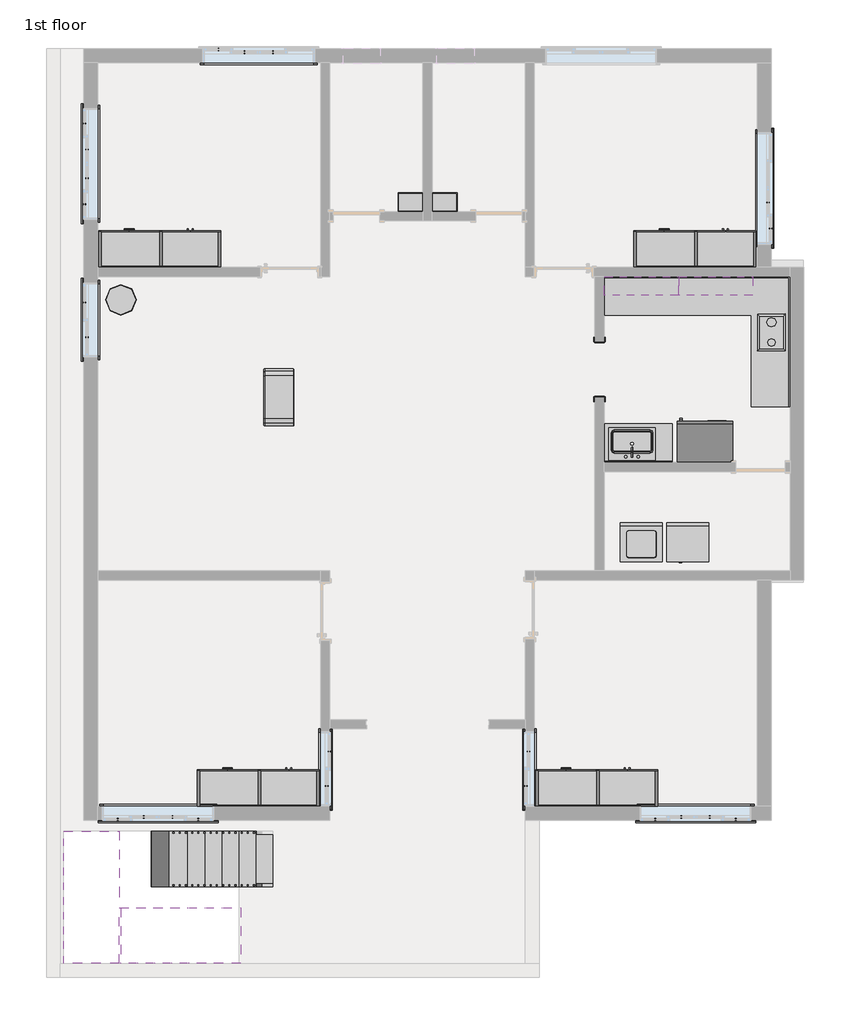
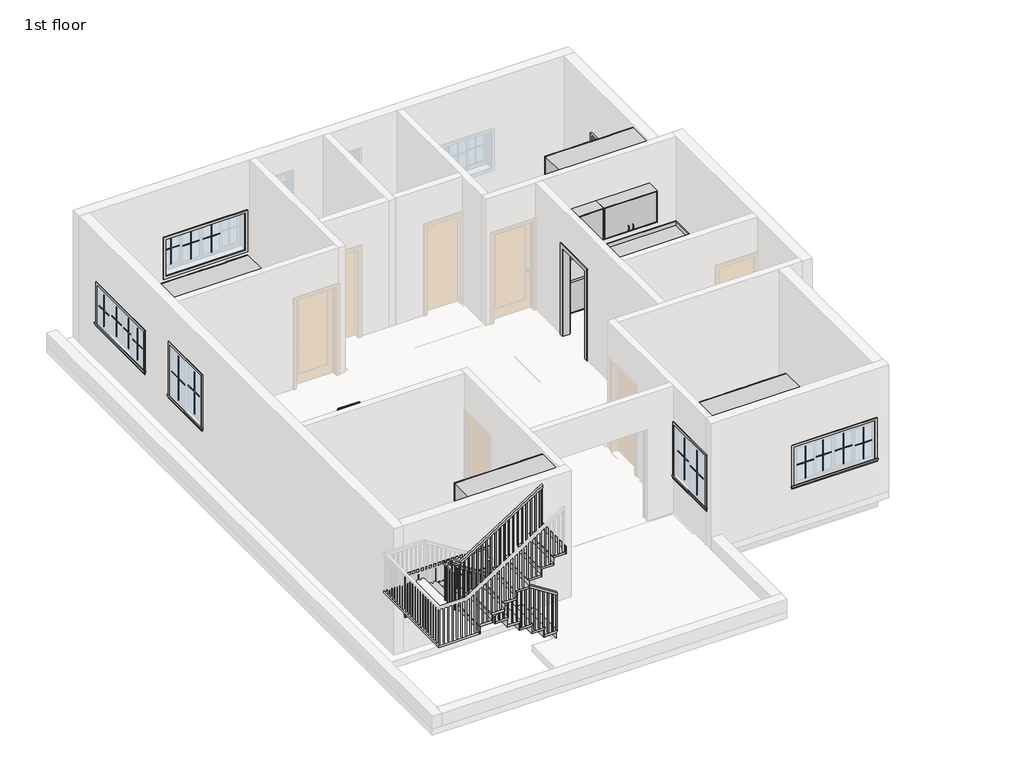
# One storey, part 3 of 4: 42 proxies, 15 furniture elements, 3 flow terminals, 2 stair flights, 1 railing, 1 slab.
"""IFC4 building model written with IfcOpenShell, lengths in millimetres."""

from ifc_helpers import new_model, si_unit, frame, origin, place, context, project, spatial, polyline, outline, extrude, faceted_brep, transform, mapped, element, save
from components import proxy_3c1fa1d0, proxy_97c73763, muntin_pattern_2x2_muntin_pattern_2x2_c2d27229, muntin_pattern_2x2_muntin_pattern_2x2_cf37b409, muntin_pattern_2x2_muntin_pattern_2x2_31a16349, proxy_7dd6dadb, trim_window_exterior_flat_with_sill_ac84ebb5, trim_window_exterior_flat_with_sill_7cfdd449, trim_window_exterior_flat_with_sill_3c945769, trim_window_interior_flat_picture_frame_caf2db4f, trim_window_interior_flat_picture_frame_f1e0b15b, trim_window_interior_flat_picture_frame_0edfbaa2, proxy_e75280ca, flow_terminal_7145266d, flow_terminal_4d548711, furniture_2dca108f, furniture_65fa61b5, furniture_1wardrobe_6271_1wardrobe_6271_4dd35231, furniture_3428e43d, furniture_bf8a676d, furniture_97fe820d, furniture_a6d59748, furniture_f5a42f9b, furniture_9d41381f, furniture_ea954fa4, non_monolithic_landing_6eacb0e7, stair_flight_6bca3b3f, stair_flight_cba1433b

model = new_model("IFC4")

# Units and contexts
model_context = context("Model", 3, world=origin())
ifc_project = project(units=[si_unit("LENGTHUNIT", "METRE", prefix="MILLI")], contexts=[model_context])

# Site, building, storey
site = spatial("IfcSite", under=ifc_project)
building = spatial("IfcBuilding", under=site)
storey = spatial("IfcBuildingStorey", under=building, Name="1st floor", Elevation=3810.0)

# Proxies
placement = place(None, origin())
proxy_shape = proxy_3c1fa1d0(model_context)
element("IfcBuildingElementProxy", 1, Name="Cook Top-2 Unit : 12\" x 18\" 2", ObjectType="Cook Top-2 Unit : 12\" x 18\" 2", at=placement, inside=storey, context=model_context, shape_type="MappedRepresentation", body=[
    mapped(proxy_shape, transform((-1440.8124084, 5502.3713848, 3810.0), x_axis=(1.0, 0.0, 0.0), y_axis=(0.0, 1.0, 0.0), z_axis=(0.0, 0.0, 1.0))),
])
proxy_2_shape = proxy_97c73763(model_context)
element("IfcBuildingElementProxy", 2, Name="Dryer : 27\" x 25\" x 35\"", ObjectType="Dryer : 27\" x 25\" x 35\"", at=placement, inside=storey, context=model_context, shape_type="MappedRepresentation", body=[
    mapped(proxy_2_shape, transform((-3115.1998647, 1776.2351766, 3810.0), x_axis=(1.0, 0.0, 0.0), y_axis=(0.0, 1.0, 0.0), z_axis=(0.0, 0.0, 1.0))),
])
muntin_pattern_2x2_muntin_pattern_2x2_shape = muntin_pattern_2x2_muntin_pattern_2x2_c2d27229(model_context)
element("IfcBuildingElementProxy", 3, Name="Muntin Pattern_2x2 : Muntin Pattern_2x2", ObjectType="Muntin Pattern_2x2 : Muntin Pattern_2x2", at=placement, inside=storey, context=model_context, shape_type="MappedRepresentation", body=[
    mapped(muntin_pattern_2x2_muntin_pattern_2x2_shape, transform((-12588.2374084, 5451.6336804, 4806.95), x_axis=(0.0, -1.0, 0.0), y_axis=(1.0, 0.0, 0.0), z_axis=(0.0, 0.0, 1.0))),
])
element("IfcBuildingElementProxy", 4, Name="Muntin Pattern_2x2 : Muntin Pattern_2x2", ObjectType="Muntin Pattern_2x2 : Muntin Pattern_2x2", at=placement, inside=storey, context=model_context, shape_type="MappedRepresentation", body=[
    mapped(muntin_pattern_2x2_muntin_pattern_2x2_shape, transform((-12632.6874084, 6019.9586804, 4806.95), x_axis=(0.0, -1.0, 0.0), y_axis=(1.0, 0.0, 0.0), z_axis=(0.0, 0.0, 1.0))),
])
muntin_pattern_2x2_muntin_pattern_2x2_2_shape = muntin_pattern_2x2_muntin_pattern_2x2_cf37b409(model_context)
element("IfcBuildingElementProxy", 5, Name="Muntin Pattern_2x2 : Muntin Pattern_2x2", ObjectType="Muntin Pattern_2x2 : Muntin Pattern_2x2", at=placement, inside=storey, context=model_context, shape_type="MappedRepresentation", body=[
    mapped(muntin_pattern_2x2_muntin_pattern_2x2_2_shape, transform((-8657.5874084, -1908.0163196, 4806.95), x_axis=(0.0, -1.0, 0.0), y_axis=(1.0, 0.0, 0.0), z_axis=(0.0, 0.0, 1.0))),
])
element("IfcBuildingElementProxy", 6, Name="Muntin Pattern_2x2 : Muntin Pattern_2x2", ObjectType="Muntin Pattern_2x2 : Muntin Pattern_2x2", at=placement, inside=storey, context=model_context, shape_type="MappedRepresentation", body=[
    mapped(muntin_pattern_2x2_muntin_pattern_2x2_2_shape, transform((-8613.1374084, -1339.6913196, 4806.95), x_axis=(0.0, -1.0, 0.0), y_axis=(1.0, 0.0, 0.0), z_axis=(0.0, 0.0, 1.0))),
])
element("IfcBuildingElementProxy", 7, Name="Muntin Pattern_2x2 : Muntin Pattern_2x2", ObjectType="Muntin Pattern_2x2 : Muntin Pattern_2x2", at=placement, inside=storey, context=model_context, shape_type="MappedRepresentation", body=[
    mapped(muntin_pattern_2x2_muntin_pattern_2x2_2_shape, transform((-5349.2374084, -1339.6913196, 4806.95), x_axis=(0.0, 1.0, 0.0), y_axis=(-1.0, 0.0, 0.0), z_axis=(0.0, 0.0, 1.0))),
])
element("IfcBuildingElementProxy", 8, Name="Muntin Pattern_2x2 : Muntin Pattern_2x2", ObjectType="Muntin Pattern_2x2 : Muntin Pattern_2x2", at=placement, inside=storey, context=model_context, shape_type="MappedRepresentation", body=[
    mapped(muntin_pattern_2x2_muntin_pattern_2x2_2_shape, transform((-5393.6874084, -1908.0163196, 4806.95), x_axis=(0.0, 1.0, 0.0), y_axis=(-1.0, 0.0, 0.0), z_axis=(0.0, 0.0, 1.0))),
])
muntin_pattern_2x2_muntin_pattern_2x2_3_shape = muntin_pattern_2x2_muntin_pattern_2x2_31a16349(model_context)
element("IfcBuildingElementProxy", 9, Name="Muntin Pattern_2x2 : Muntin Pattern_2x2", ObjectType="Muntin Pattern_2x2 : Muntin Pattern_2x2", at=placement, inside=storey, context=model_context, shape_type="MappedRepresentation", body=[
    mapped(muntin_pattern_2x2_muntin_pattern_2x2_3_shape, transform((-10432.4124084, 10171.2711804, 4806.95), x_axis=(1.0, 0.0, 0.0), y_axis=(0.0, 1.0, 0.0), z_axis=(0.0, 0.0, 1.0))),
])
element("IfcBuildingElementProxy", 10, Name="Muntin Pattern_2x2 : Muntin Pattern_2x2", ObjectType="Muntin Pattern_2x2 : Muntin Pattern_2x2", at=placement, inside=storey, context=model_context, shape_type="MappedRepresentation", body=[
    mapped(muntin_pattern_2x2_muntin_pattern_2x2_3_shape, transform((-10006.9624084, 10126.8211804, 4806.95), x_axis=(1.0, 0.0, 0.0), y_axis=(0.0, 1.0, 0.0), z_axis=(0.0, 0.0, 1.0))),
])
element("IfcBuildingElementProxy", 11, Name="Muntin Pattern_2x2 : Muntin Pattern_2x2", ObjectType="Muntin Pattern_2x2 : Muntin Pattern_2x2", at=placement, inside=storey, context=model_context, shape_type="MappedRepresentation", body=[
    mapped(muntin_pattern_2x2_muntin_pattern_2x2_3_shape, transform((-9537.0624084, 10126.8211804, 4806.95), x_axis=(1.0, 0.0, 0.0), y_axis=(0.0, 1.0, 0.0), z_axis=(0.0, 0.0, 1.0))),
])
element("IfcBuildingElementProxy", 12, Name="Muntin Pattern_2x2 : Muntin Pattern_2x2", ObjectType="Muntin Pattern_2x2 : Muntin Pattern_2x2", at=placement, inside=storey, context=model_context, shape_type="MappedRepresentation", body=[
    mapped(muntin_pattern_2x2_muntin_pattern_2x2_3_shape, transform((-12632.6874084, 7634.4461804, 4806.95), x_axis=(0.0, 1.0, 0.0), y_axis=(-1.0, 0.0, 0.0), z_axis=(0.0, 0.0, 1.0))),
])
element("IfcBuildingElementProxy", 13, Name="Muntin Pattern_2x2 : Muntin Pattern_2x2", ObjectType="Muntin Pattern_2x2 : Muntin Pattern_2x2", at=placement, inside=storey, context=model_context, shape_type="MappedRepresentation", body=[
    mapped(muntin_pattern_2x2_muntin_pattern_2x2_3_shape, transform((-12588.2374084, 8059.8961804, 4806.95), x_axis=(0.0, 1.0, 0.0), y_axis=(-1.0, 0.0, 0.0), z_axis=(0.0, 0.0, 1.0))),
])
element("IfcBuildingElementProxy", 14, Name="Muntin Pattern_2x2 : Muntin Pattern_2x2", ObjectType="Muntin Pattern_2x2 : Muntin Pattern_2x2", at=placement, inside=storey, context=model_context, shape_type="MappedRepresentation", body=[
    mapped(muntin_pattern_2x2_muntin_pattern_2x2_3_shape, transform((-12588.2374084, 8529.7961804, 4806.95), x_axis=(0.0, 1.0, 0.0), y_axis=(-1.0, 0.0, 0.0), z_axis=(0.0, 0.0, 1.0))),
])
element("IfcBuildingElementProxy", 15, Name="Muntin Pattern_2x2 : Muntin Pattern_2x2", ObjectType="Muntin Pattern_2x2 : Muntin Pattern_2x2", at=placement, inside=storey, context=model_context, shape_type="MappedRepresentation", body=[
    mapped(muntin_pattern_2x2_muntin_pattern_2x2_3_shape, transform((-12632.6874084, 8955.2461804, 4806.95), x_axis=(0.0, 1.0, 0.0), y_axis=(-1.0, 0.0, 0.0), z_axis=(0.0, 0.0, 1.0))),
])
element("IfcBuildingElementProxy", 16, Name="Muntin Pattern_2x2 : Muntin Pattern_2x2", ObjectType="Muntin Pattern_2x2 : Muntin Pattern_2x2", at=placement, inside=storey, context=model_context, shape_type="MappedRepresentation", body=[
    mapped(muntin_pattern_2x2_muntin_pattern_2x2_3_shape, transform((-1418.5874084, 7659.8461804, 4806.95), x_axis=(0.0, -1.0, 0.0), y_axis=(1.0, 0.0, 0.0), z_axis=(0.0, 0.0, 1.0))),
])
element("IfcBuildingElementProxy", 17, Name="Muntin Pattern_2x2 : Muntin Pattern_2x2", ObjectType="Muntin Pattern_2x2 : Muntin Pattern_2x2", at=placement, inside=storey, context=model_context, shape_type="MappedRepresentation", body=[
    mapped(muntin_pattern_2x2_muntin_pattern_2x2_3_shape, transform((-1374.1374084, 7234.3961804, 4806.95), x_axis=(0.0, -1.0, 0.0), y_axis=(1.0, 0.0, 0.0), z_axis=(0.0, 0.0, 1.0))),
])
element("IfcBuildingElementProxy", 18, Name="Muntin Pattern_2x2 : Muntin Pattern_2x2", ObjectType="Muntin Pattern_2x2 : Muntin Pattern_2x2", at=placement, inside=storey, context=model_context, shape_type="MappedRepresentation", body=[
    mapped(muntin_pattern_2x2_muntin_pattern_2x2_3_shape, transform((-1948.8124084, -2458.8788196, 4806.95), x_axis=(-1.0, 0.0, 0.0), y_axis=(0.0, -1.0, 0.0), z_axis=(0.0, 0.0, 1.0))),
])
element("IfcBuildingElementProxy", 19, Name="Muntin Pattern_2x2 : Muntin Pattern_2x2", ObjectType="Muntin Pattern_2x2 : Muntin Pattern_2x2", at=placement, inside=storey, context=model_context, shape_type="MappedRepresentation", body=[
    mapped(muntin_pattern_2x2_muntin_pattern_2x2_3_shape, transform((-2374.2624084, -2414.4288196, 4806.95), x_axis=(-1.0, 0.0, 0.0), y_axis=(0.0, -1.0, 0.0), z_axis=(0.0, 0.0, 1.0))),
])
element("IfcBuildingElementProxy", 20, Name="Muntin Pattern_2x2 : Muntin Pattern_2x2", ObjectType="Muntin Pattern_2x2 : Muntin Pattern_2x2", at=placement, inside=storey, context=model_context, shape_type="MappedRepresentation", body=[
    mapped(muntin_pattern_2x2_muntin_pattern_2x2_3_shape, transform((-2844.1624084, -2414.4288196, 4806.95), x_axis=(-1.0, 0.0, 0.0), y_axis=(0.0, -1.0, 0.0), z_axis=(0.0, 0.0, 1.0))),
])
element("IfcBuildingElementProxy", 21, Name="Muntin Pattern_2x2 : Muntin Pattern_2x2", ObjectType="Muntin Pattern_2x2 : Muntin Pattern_2x2", at=placement, inside=storey, context=model_context, shape_type="MappedRepresentation", body=[
    mapped(muntin_pattern_2x2_muntin_pattern_2x2_3_shape, transform((-3269.6124084, -2458.8788196, 4806.95), x_axis=(-1.0, 0.0, 0.0), y_axis=(0.0, -1.0, 0.0), z_axis=(0.0, 0.0, 1.0))),
])
element("IfcBuildingElementProxy", 22, Name="Muntin Pattern_2x2 : Muntin Pattern_2x2", ObjectType="Muntin Pattern_2x2 : Muntin Pattern_2x2", at=placement, inside=storey, context=model_context, shape_type="MappedRepresentation", body=[
    mapped(muntin_pattern_2x2_muntin_pattern_2x2_3_shape, transform((-10762.6124084, -2458.8788196, 4806.95), x_axis=(-1.0, 0.0, 0.0), y_axis=(0.0, -1.0, 0.0), z_axis=(0.0, 0.0, 1.0))),
])
element("IfcBuildingElementProxy", 23, Name="Muntin Pattern_2x2 : Muntin Pattern_2x2", ObjectType="Muntin Pattern_2x2 : Muntin Pattern_2x2", at=placement, inside=storey, context=model_context, shape_type="MappedRepresentation", body=[
    mapped(muntin_pattern_2x2_muntin_pattern_2x2_3_shape, transform((-11188.0624084, -2414.4288196, 4806.95), x_axis=(-1.0, 0.0, 0.0), y_axis=(0.0, -1.0, 0.0), z_axis=(0.0, 0.0, 1.0))),
])
element("IfcBuildingElementProxy", 24, Name="Muntin Pattern_2x2 : Muntin Pattern_2x2", ObjectType="Muntin Pattern_2x2 : Muntin Pattern_2x2", at=placement, inside=storey, context=model_context, shape_type="MappedRepresentation", body=[
    mapped(muntin_pattern_2x2_muntin_pattern_2x2_3_shape, transform((-11657.9624084, -2414.4288196, 4806.95), x_axis=(-1.0, 0.0, 0.0), y_axis=(0.0, -1.0, 0.0), z_axis=(0.0, 0.0, 1.0))),
])
element("IfcBuildingElementProxy", 25, Name="Muntin Pattern_2x2 : Muntin Pattern_2x2", ObjectType="Muntin Pattern_2x2 : Muntin Pattern_2x2", at=placement, inside=storey, context=model_context, shape_type="MappedRepresentation", body=[
    mapped(muntin_pattern_2x2_muntin_pattern_2x2_3_shape, transform((-12083.4124084, -2458.8788196, 4806.95), x_axis=(-1.0, 0.0, 0.0), y_axis=(0.0, -1.0, 0.0), z_axis=(0.0, 0.0, 1.0))),
])
proxy_3_shape = proxy_7dd6dadb(model_context)
element("IfcBuildingElementProxy", 26, Name="Passage Opening-Cased : 36\" x 84\"", ObjectType="Passage Opening-Cased : 36\" x 84\"", at=placement, inside=storey, context=model_context, shape_type="MappedRepresentation", body=[
    mapped(proxy_3_shape, transform((-4184.0124084, 4931.1848371, 3810.0), x_axis=(0.0, 1.0, 0.0), y_axis=(-1.0, 0.0, 0.0), z_axis=(0.0, 0.0, 1.0))),
])
trim_window_exterior_flat_with_sill_shape = trim_window_exterior_flat_with_sill_ac84ebb5(model_context)
element("IfcBuildingElementProxy", 27, Name="Trim-Window-Exterior-Flat : with Sill", ObjectType="Trim-Window-Exterior-Flat : with Sill", at=placement, inside=storey, context=model_context, shape_type="MappedRepresentation", body=[
    mapped(trim_window_exterior_flat_with_sill_shape, transform((-12642.2124084, 5735.7961804, 5943.6), x_axis=(0.0, 1.0, 0.0), y_axis=(0.0, 0.0, -1.0), z_axis=(-1.0, 0.0, 0.0))),
])
trim_window_exterior_flat_with_sill_2_shape = trim_window_exterior_flat_with_sill_7cfdd449(model_context)
element("IfcBuildingElementProxy", 28, Name="Trim-Window-Exterior-Flat : with Sill", ObjectType="Trim-Window-Exterior-Flat : with Sill", at=placement, inside=storey, context=model_context, shape_type="MappedRepresentation", body=[
    mapped(trim_window_exterior_flat_with_sill_2_shape, transform((-8603.6124084, -1623.8538196, 5943.6), x_axis=(0.0, 1.0, 0.0), y_axis=(0.0, 0.0, 1.0), z_axis=(1.0, 0.0, 0.0))),
])
element("IfcBuildingElementProxy", 29, Name="Trim-Window-Exterior-Flat : with Sill", ObjectType="Trim-Window-Exterior-Flat : with Sill", at=placement, inside=storey, context=model_context, shape_type="MappedRepresentation", body=[
    mapped(trim_window_exterior_flat_with_sill_2_shape, transform((-5403.2124084, -1623.8538196, 5943.6), x_axis=(0.0, -1.0, 0.0), y_axis=(0.0, 0.0, 1.0), z_axis=(-1.0, 0.0, 0.0))),
])
trim_window_exterior_flat_with_sill_3_shape = trim_window_exterior_flat_with_sill_3c945769(model_context)
element("IfcBuildingElementProxy", 30, Name="Trim-Window-Exterior-Flat : with Sill", ObjectType="Trim-Window-Exterior-Flat : with Sill", at=placement, inside=storey, context=model_context, shape_type="MappedRepresentation", body=[
    mapped(trim_window_exterior_flat_with_sill_3_shape, transform((-12642.2124084, 8294.8461804, 5638.8), x_axis=(0.0, -1.0, 0.0), y_axis=(0.0, 0.0, 1.0), z_axis=(-1.0, 0.0, 0.0))),
])
element("IfcBuildingElementProxy", 31, Name="Trim-Window-Exterior-Flat : with Sill", ObjectType="Trim-Window-Exterior-Flat : with Sill", at=placement, inside=storey, context=model_context, shape_type="MappedRepresentation", body=[
    mapped(trim_window_exterior_flat_with_sill_3_shape, transform((-1364.6124084, 7894.7961804, 5638.8), x_axis=(0.0, 1.0, 0.0), y_axis=(0.0, 0.0, 1.0), z_axis=(1.0, 0.0, 0.0))),
])
element("IfcBuildingElementProxy", 32, Name="Trim-Window-Exterior-Flat : with Sill", ObjectType="Trim-Window-Exterior-Flat : with Sill", at=placement, inside=storey, context=model_context, shape_type="MappedRepresentation", body=[
    mapped(trim_window_exterior_flat_with_sill_3_shape, transform((-2609.2124084, -2468.4038196, 5638.8), x_axis=(1.0, 0.0, 0.0), y_axis=(0.0, 0.0, 1.0), z_axis=(0.0, -1.0, 0.0))),
])
element("IfcBuildingElementProxy", 33, Name="Trim-Window-Exterior-Flat : with Sill", ObjectType="Trim-Window-Exterior-Flat : with Sill", at=placement, inside=storey, context=model_context, shape_type="MappedRepresentation", body=[
    mapped(trim_window_exterior_flat_with_sill_3_shape, transform((-11423.0124084, -2468.4038196, 5638.8), x_axis=(1.0, 0.0, 0.0), y_axis=(0.0, 0.0, 1.0), z_axis=(0.0, -1.0, 0.0))),
])
trim_window_interior_flat_picture_frame_shape = trim_window_interior_flat_picture_frame_caf2db4f(model_context)
element("IfcBuildingElementProxy", 34, Name="Trim-Window-Interior-Flat : Picture Frame", ObjectType="Trim-Window-Interior-Flat : Picture Frame", at=placement, inside=storey, context=model_context, shape_type="MappedRepresentation", body=[
    mapped(trim_window_interior_flat_picture_frame_shape, transform((-12413.6124084, 5735.7961804, 5943.6), x_axis=(0.0, -1.0, 0.0), y_axis=(0.0, 0.0, -1.0), z_axis=(1.0, 0.0, 0.0))),
])
trim_window_interior_flat_picture_frame_2_shape = trim_window_interior_flat_picture_frame_f1e0b15b(model_context)
element("IfcBuildingElementProxy", 35, Name="Trim-Window-Interior-Flat : Picture Frame", ObjectType="Trim-Window-Interior-Flat : Picture Frame", at=placement, inside=storey, context=model_context, shape_type="MappedRepresentation", body=[
    mapped(trim_window_interior_flat_picture_frame_2_shape, transform((-8756.0124084, -1623.8538196, 5943.6), x_axis=(0.0, -1.0, 0.0), y_axis=(0.0, 0.0, 1.0), z_axis=(-1.0, 0.0, 0.0))),
])
element("IfcBuildingElementProxy", 36, Name="Trim-Window-Interior-Flat : Picture Frame", ObjectType="Trim-Window-Interior-Flat : Picture Frame", at=placement, inside=storey, context=model_context, shape_type="MappedRepresentation", body=[
    mapped(trim_window_interior_flat_picture_frame_2_shape, transform((-5250.8124084, -1623.8538196, 5943.6), x_axis=(0.0, 1.0, 0.0), y_axis=(0.0, 0.0, 1.0), z_axis=(1.0, 0.0, 0.0))),
])
trim_window_interior_flat_picture_frame_3_shape = trim_window_interior_flat_picture_frame_0edfbaa2(model_context)
element("IfcBuildingElementProxy", 37, Name="Trim-Window-Interior-Flat : Picture Frame", ObjectType="Trim-Window-Interior-Flat : Picture Frame", at=placement, inside=storey, context=model_context, shape_type="MappedRepresentation", body=[
    mapped(trim_window_interior_flat_picture_frame_3_shape, transform((-9772.0124084, 9952.1961804, 5638.8), x_axis=(1.0, 0.0, 0.0), y_axis=(0.0, 0.0, 1.0), z_axis=(0.0, -1.0, 0.0))),
])
element("IfcBuildingElementProxy", 38, Name="Trim-Window-Interior-Flat : Picture Frame", ObjectType="Trim-Window-Interior-Flat : Picture Frame", at=placement, inside=storey, context=model_context, shape_type="MappedRepresentation", body=[
    mapped(trim_window_interior_flat_picture_frame_3_shape, transform((-12413.6124084, 8294.8461804, 5638.8), x_axis=(0.0, 1.0, 0.0), y_axis=(0.0, 0.0, 1.0), z_axis=(1.0, 0.0, 0.0))),
])
element("IfcBuildingElementProxy", 39, Name="Trim-Window-Interior-Flat : Picture Frame", ObjectType="Trim-Window-Interior-Flat : Picture Frame", at=placement, inside=storey, context=model_context, shape_type="MappedRepresentation", body=[
    mapped(trim_window_interior_flat_picture_frame_3_shape, transform((-1593.2124084, 7894.7961804, 5638.8), x_axis=(0.0, -1.0, 0.0), y_axis=(0.0, 0.0, 1.0), z_axis=(-1.0, 0.0, 0.0))),
])
element("IfcBuildingElementProxy", 40, Name="Trim-Window-Interior-Flat : Picture Frame", ObjectType="Trim-Window-Interior-Flat : Picture Frame", at=placement, inside=storey, context=model_context, shape_type="MappedRepresentation", body=[
    mapped(trim_window_interior_flat_picture_frame_3_shape, transform((-2609.2124084, -2239.8038196, 5638.8), x_axis=(-1.0, 0.0, 0.0), y_axis=(0.0, 0.0, 1.0), z_axis=(0.0, 1.0, 0.0))),
])
element("IfcBuildingElementProxy", 41, Name="Trim-Window-Interior-Flat : Picture Frame", ObjectType="Trim-Window-Interior-Flat : Picture Frame", at=placement, inside=storey, context=model_context, shape_type="MappedRepresentation", body=[
    mapped(trim_window_interior_flat_picture_frame_3_shape, transform((-11423.0124084, -2239.8038196, 5638.8), x_axis=(-1.0, 0.0, 0.0), y_axis=(0.0, 0.0, 1.0), z_axis=(0.0, 1.0, 0.0))),
])
proxy_4_shape = proxy_e75280ca(model_context)
element("IfcBuildingElementProxy", 42, Name="Washer : 27\" x 25\" x 35\"", ObjectType="Washer : 27\" x 25\" x 35\"", at=placement, inside=storey, context=model_context, shape_type="MappedRepresentation", body=[
    mapped(proxy_4_shape, transform((-3918.6298768, 1811.7466156, 3810.0), x_axis=(1.0, 0.0, 0.0), y_axis=(0.0, 1.0, 0.0), z_axis=(0.0, 0.0, 1.0))),
])

# Flow terminals
flow_terminal_shape = flow_terminal_7145266d(model_context)
element("IfcFlowTerminal", 43, ObjectType="Sink - Work : 20\"x18\" 2", at=placement, inside=storey, context=model_context, shape_type="MappedRepresentation", body=[
    mapped(flow_terminal_shape, transform((-7282.8124084, 7513.7961804, 4724.4), x_axis=(-1.0, 0.0, 0.0), y_axis=(0.0, -1.0, 0.0), z_axis=(0.0, 0.0, 1.0))),
])
element("IfcFlowTerminal", 44, ObjectType="Sink - Work : 20\"x18\" 2", at=placement, inside=storey, context=model_context, shape_type="MappedRepresentation", body=[
    mapped(flow_terminal_shape, transform((-6724.0124084, 7513.7961804, 4724.4), x_axis=(-1.0, 0.0, 0.0), y_axis=(0.0, -1.0, 0.0), z_axis=(0.0, 0.0, 1.0))),
])
flow_terminal_2_shape = flow_terminal_4d548711(model_context)
element("IfcFlowTerminal", 45, ObjectType="Sink Kitchen-Single : 30\" x 21\"", at=placement, inside=storey, context=model_context, shape_type="MappedRepresentation", body=[
    mapped(flow_terminal_2_shape, transform((-3634.9231678, 3706.1415815, 3810.0), x_axis=(-1.0, 0.0, 0.0), y_axis=(0.0, -1.0, 0.0), z_axis=(0.0, 0.0, 1.0))),
])

# Furniture
furniture_shape = furniture_2dca108f(model_context)
element("IfcFurniture", 46, at=placement, inside=storey, context=model_context, shape_type="MappedRepresentation", body=[
    mapped(furniture_shape, transform((-9441.8124084, 4465.7961804, 3810.0), x_axis=(1.0, 0.0, 0.0), y_axis=(0.0, 1.0, 0.0), z_axis=(0.0, 0.0, 1.0))),
])
furniture_2_shape = furniture_65fa61b5(model_context)
element("IfcFurniture", 47, at=placement, inside=storey, context=model_context, shape_type="MappedRepresentation", body=[
    mapped(furniture_2_shape, transform((-3066.4124084, 3411.6961804, 3810.0), x_axis=(-1.0, 0.0, 0.0), y_axis=(0.0, -1.0, 0.0), z_axis=(0.0, 0.0, 1.0))),
])
furniture_1wardrobe_6271_1wardrobe_6271_shape = furniture_1wardrobe_6271_1wardrobe_6271_4dd35231(model_context)
element("IfcFurniture", 48, ObjectType="1Wardrobe_6271 : 1Wardrobe_6271", at=placement, inside=storey, context=model_context, shape_type="MappedRepresentation", body=[
    mapped(furniture_1wardrobe_6271_1wardrobe_6271_shape, transform((-10394.3124084, 6599.3961804, 3810.0), x_axis=(-1.0, 0.0, 0.0), y_axis=(0.0, -1.0, 0.0), z_axis=(0.0, 0.0, 1.0))),
])
element("IfcFurniture", 49, ObjectType="1Wardrobe_6271 : 1Wardrobe_6271", at=placement, inside=storey, context=model_context, shape_type="MappedRepresentation", body=[
    mapped(furniture_1wardrobe_6271_1wardrobe_6271_shape, transform((-1618.6124084, 6599.3961804, 3810.0), x_axis=(-1.0, 0.0, 0.0), y_axis=(0.0, -1.0, 0.0), z_axis=(0.0, 0.0, 1.0))),
])
element("IfcFurniture", 50, ObjectType="1Wardrobe_6271 : 1Wardrobe_6271", at=placement, inside=storey, context=model_context, shape_type="MappedRepresentation", body=[
    mapped(furniture_1wardrobe_6271_1wardrobe_6271_shape, transform((-3231.5124084, -2239.8038196, 3810.0), x_axis=(-1.0, 0.0, 0.0), y_axis=(0.0, -1.0, 0.0), z_axis=(0.0, 0.0, 1.0))),
])
element("IfcFurniture", 51, ObjectType="1Wardrobe_6271 : 1Wardrobe_6271", at=placement, inside=storey, context=model_context, shape_type="MappedRepresentation", body=[
    mapped(furniture_1wardrobe_6271_1wardrobe_6271_shape, transform((-8781.4124084, -2239.8038196, 3810.0), x_axis=(-1.0, 0.0, 0.0), y_axis=(0.0, -1.0, 0.0), z_axis=(0.0, 0.0, 1.0))),
])
furniture_3_shape = furniture_3428e43d(model_context)
element("IfcFurniture", 52, ObjectType="48\" 2", at=placement, inside=storey, context=model_context, shape_type="MappedRepresentation", body=[
    mapped(furniture_3_shape, transform((-2674.6573683, 6446.9961804, 3810.0), x_axis=(1.0, 0.0, 0.0), y_axis=(0.0, 1.0, 0.0), z_axis=(0.0, 0.0, 1.0))),
])
element("IfcFurniture", 53, ObjectType="48\" 3", at=placement, inside=storey, context=model_context, shape_type="MappedRepresentation", body=[
    mapped(furniture_3_shape, transform((-1059.8124084, 5013.8411403, 3810.0), x_axis=(0.0, -1.0, 0.0), y_axis=(1.0, 0.0, 0.0), z_axis=(0.0, 0.0, 1.0))),
])
furniture_4_shape = furniture_bf8a676d(model_context)
element("IfcFurniture", 54, ObjectType="Base Cabinet-Combo01 : 30\" 2", at=placement, inside=storey, context=model_context, shape_type="MappedRepresentation", body=[
    mapped(furniture_4_shape, transform((-3669.3501133, 6446.9961804, 3810.0), x_axis=(1.0, 0.0, 0.0), y_axis=(0.0, 1.0, 0.0), z_axis=(0.0, 0.0, 1.0))),
])
furniture_5_shape = furniture_97fe820d(model_context)
element("IfcFurniture", 55, ObjectType="Base Cabinet-Corner Unit-Square : 36\"", at=placement, inside=storey, context=model_context, shape_type="MappedRepresentation", body=[
    mapped(furniture_5_shape, transform((-1586.5501133, 6446.9961804, 3810.0), x_axis=(1.0, 0.0, 0.0), y_axis=(0.0, 1.0, 0.0), z_axis=(0.0, 0.0, 1.0))),
])
furniture_6_shape = furniture_a6d59748(model_context)
element("IfcFurniture", 56, ObjectType="Counter Top w Sink Hole : 24\" Depth", at=placement, inside=storey, context=model_context, shape_type="MappedRepresentation", body=[
    mapped(furniture_6_shape, transform((-4190.6747034, 3398.9961804, 3810.0), x_axis=(-1.0, 0.0, 0.0), y_axis=(0.0, -1.0, 0.0), z_axis=(0.0, 0.0, 1.0))),
])
furniture_7_shape = furniture_f5a42f9b(model_context)
element("IfcFurniture", 57, ObjectType="Counter Top-L Shaped : 24\" Depth", at=placement, inside=storey, context=model_context, shape_type="MappedRepresentation", body=[
    mapped(furniture_7_shape, transform((-1059.8124084, 5246.5338853, 3810.0), x_axis=(0.0, -1.0, 0.0), y_axis=(1.0, 0.0, 0.0), z_axis=(0.0, 0.0, 1.0))),
])
furniture_8_shape = furniture_9d41381f(model_context)
element("IfcFurniture", 58, ObjectType="Table-Trio End : 20\" Diameter", at=placement, inside=storey, context=model_context, shape_type="MappedRepresentation", body=[
    mapped(furniture_8_shape, transform((-12032.6124084, 6065.9961804, 3810.0), x_axis=(1.0, 0.0, 0.0), y_axis=(0.0, 1.0, 0.0), z_axis=(0.0, 0.0, 1.0))),
])
furniture_9_shape = furniture_ea954fa4(model_context)
element("IfcFurniture", 59, ObjectType="Upper Cabinet-Pass-Thru : 48\" x 30\" x 12\"", at=placement, inside=storey, context=model_context, shape_type="MappedRepresentation", body=[
    mapped(furniture_9_shape, transform((-3516.9501133, 6446.9961804, 3810.0), x_axis=(1.0, 0.0, 0.0), y_axis=(0.0, 1.0, 0.0), z_axis=(0.0, 0.0, 1.0))),
])
element("IfcFurniture", 60, ObjectType="Upper Cabinet-Pass-Thru : 48\" x 30\" x 12\"", at=placement, inside=storey, context=model_context, shape_type="MappedRepresentation", body=[
    mapped(furniture_9_shape, transform((-2297.7501133, 6446.9961804, 3810.0), x_axis=(1.0, 0.0, 0.0), y_axis=(0.0, 1.0, 0.0), z_axis=(0.0, 0.0, 1.0))),
])

# Railing
element("IfcRailing", 61, ObjectType="Handrail - Rectangular", at=placement, inside=storey, context=model_context, shape_type="SolidModel", body=[
    faceted_brep([(-9543.8120641, -3562.3669819, 4902.2), (-9543.8120641, -3562.3669819, 4841.986276), (-9543.8120641, -3511.5669819, 4841.986276), (-9543.8120641, -3511.5669819, 4902.2), (-11982.2120641, -3562.3669819, 6453.9090909), (-12033.0120641, -3562.3669819, 6426.0226396), (-12033.0120641, -3511.5669819, 6426.0226396), (-11982.2120641, -3511.5669819, 6453.9090909), (-11982.2120641, -3562.3669819, 6502.4), (-12033.0120641, -3562.3669819, 6451.6), (-12033.0120641, -3511.5669819, 6451.6), (-11982.2120641, -3511.5669819, 6502.4), (-12058.4120641, -3562.3669819, 6502.4), (-12058.4120641, -3562.3669819, 6451.6), (-12109.2120641, -3511.5669819, 6451.6), (-12109.2120641, -3511.5669819, 6502.4), (-12058.4120641, -3638.5669819, 6502.4), (-12058.4120641, -3638.5669819, 6451.6), (-12109.2120641, -3638.5669819, 6451.6), (-12109.2120641, -3638.5669819, 6502.4), (-12058.4120641, -3827.3038196, 6502.4), (-12058.4120641, -3878.1038196, 6451.6), (-12109.2120641, -3878.1038196, 6451.6), (-12109.2120641, -3827.3038196, 6502.4), (-12058.4120641, -3827.3038196, 6728.6909091), (-12058.4120641, -3878.1038196, 6677.8909091), (-12109.2120641, -3878.1038196, 6677.8909091), (-12109.2120641, -3827.3038196, 6728.6909091), (-12058.4120641, -3903.5038196, 6728.6909091), (-12058.4120641, -3903.5038196, 6677.8909091), (-12109.2120641, -3954.3038196, 6677.8909091), (-12109.2120641, -3954.3038196, 6728.6909091), (-11982.2120641, -3903.5038196, 6728.6909091), (-11967.4190691, -3903.5038196, 6677.8909091), (-11967.4190691, -3954.3038196, 6677.8909091), (-11982.2120641, -3954.3038196, 6728.6909091), (-10102.6120641, -3903.5038196, 7924.8), (-10102.6120641, -3954.3038196, 7924.8), (-10102.6120641, -3954.3038196, 7864.586276), (-10102.6120641, -3903.5038196, 7864.586276)], [[[0, 1, 2, 3]], [[1, 0, 4, 5]], [[2, 1, 5, 6]], [[3, 2, 6, 7]], [[0, 3, 7, 4]], [[5, 4, 8, 9]], [[6, 5, 9, 10]], [[7, 6, 10, 11]], [[4, 7, 11, 8]], [[9, 8, 12, 13]], [[10, 9, 13, 14]], [[11, 10, 14, 15]], [[8, 11, 15, 12]], [[13, 12, 16, 17]], [[14, 13, 17, 18]], [[15, 14, 18, 19]], [[12, 15, 19, 16]], [[17, 16, 20, 21]], [[18, 17, 21, 22]], [[19, 18, 22, 23]], [[16, 19, 23, 20]], [[21, 20, 24, 25]], [[22, 21, 25, 26]], [[23, 22, 26, 27]], [[20, 23, 27, 24]], [[25, 24, 28, 29]], [[26, 25, 29, 30]], [[27, 26, 30, 31]], [[24, 27, 31, 28]], [[29, 28, 32, 33]], [[30, 29, 33, 34]], [[31, 30, 34, 35]], [[28, 31, 35, 32]], [[36, 37, 38, 39]], [[33, 32, 36, 39]], [[34, 33, 39, 38]], [[35, 34, 38, 37]], [[32, 35, 37, 36]]]),
    extrude(outline(polyline([(7826.1976396, -10162.9370641), (6832.6, -10162.9370641), (6832.6, -10143.8870641), (7838.3203669, -10143.8870641), (7826.1976396, -10162.9370641)])), frame((0.0, -3938.4288196, 0.0), z_axis=(0.0, 1.0, 0.0), x_axis=(0.0, 0.0, 1.0)), (0.0, 0.0, 1.0), 19.05),
    extrude(outline(polyline([(7761.5430941, -10264.5370641), (6832.6, -10264.5370641), (6832.6, -10245.4870641), (7773.6658214, -10245.4870641), (7761.5430941, -10264.5370641)])), frame((0.0, -3938.4288196, 0.0), z_axis=(0.0, 1.0, 0.0), x_axis=(0.0, 0.0, 1.0)), (0.0, 0.0, 1.0), 19.05),
    extrude(outline(polyline([(7696.8885487, -10366.1370641), (6832.6, -10366.1370641), (6832.6, -10347.0870641), (7709.011276, -10347.0870641), (7696.8885487, -10366.1370641)])), frame((0.0, -3938.4288196, 0.0), z_axis=(0.0, 1.0, 0.0), x_axis=(0.0, 0.0, 1.0)), (0.0, 0.0, 1.0), 19.05),
    extrude(outline(polyline([(7632.2340032, -10467.7370641), (6654.8, -10467.7370641), (6654.8, -10448.6870641), (7644.3567305, -10448.6870641), (7632.2340032, -10467.7370641)])), frame((0.0, -3938.4288196, 0.0), z_axis=(0.0, 1.0, 0.0), x_axis=(0.0, 0.0, 1.0)), (0.0, 0.0, 1.0), 19.05),
    extrude(outline(polyline([(7567.5794578, -10569.3370641), (6654.8, -10569.3370641), (6654.8, -10550.2870641), (7579.7021851, -10550.2870641), (7567.5794578, -10569.3370641)])), frame((0.0, -3938.4288196, 0.0), z_axis=(0.0, 1.0, 0.0), x_axis=(0.0, 0.0, 1.0)), (0.0, 0.0, 1.0), 19.05),
    extrude(outline(polyline([(7502.9249123, -10670.9370641), (6654.8, -10670.9370641), (6654.8, -10651.8870641), (7515.0476396, -10651.8870641), (7502.9249123, -10670.9370641)])), frame((0.0, -3938.4288196, 0.0), z_axis=(0.0, 1.0, 0.0), x_axis=(0.0, 0.0, 1.0)), (0.0, 0.0, 1.0), 19.05),
    extrude(outline(polyline([(7438.2703669, -10772.5370641), (6477.0, -10772.5370641), (6477.0, -10753.4870641), (7450.3930941, -10753.4870641), (7438.2703669, -10772.5370641)])), frame((0.0, -3938.4288196, 0.0), z_axis=(0.0, 1.0, 0.0), x_axis=(0.0, 0.0, 1.0)), (0.0, 0.0, 1.0), 19.05),
    extrude(outline(polyline([(7373.6158214, -10874.1370641), (6477.0, -10874.1370641), (6477.0, -10855.0870641), (7385.7385487, -10855.0870641), (7373.6158214, -10874.1370641)])), frame((0.0, -3938.4288196, 0.0), z_axis=(0.0, 1.0, 0.0), x_axis=(0.0, 0.0, 1.0)), (0.0, 0.0, 1.0), 19.05),
    extrude(outline(polyline([(7308.961276, -10975.7370641), (6299.2, -10975.7370641), (6299.2, -10956.6870641), (7321.0840032, -10956.6870641), (7308.961276, -10975.7370641)])), frame((0.0, -3938.4288196, 0.0), z_axis=(0.0, 1.0, 0.0), x_axis=(0.0, 0.0, 1.0)), (0.0, 0.0, 1.0), 19.05),
    extrude(outline(polyline([(7244.3067305, -11077.3370641), (6299.2, -11077.3370641), (6299.2, -11058.2870641), (7256.4294578, -11058.2870641), (7244.3067305, -11077.3370641)])), frame((0.0, -3938.4288196, 0.0), z_axis=(0.0, 1.0, 0.0), x_axis=(0.0, 0.0, 1.0)), (0.0, 0.0, 1.0), 19.05),
    extrude(outline(polyline([(7179.6521851, -11178.9370641), (6299.2, -11178.9370641), (6299.2, -11159.8870641), (7191.7749123, -11159.8870641), (7179.6521851, -11178.9370641)])), frame((0.0, -3938.4288196, 0.0), z_axis=(0.0, 1.0, 0.0), x_axis=(0.0, 0.0, 1.0)), (0.0, 0.0, 1.0), 19.05),
    extrude(outline(polyline([(7114.9976396, -11280.5370641), (6121.4, -11280.5370641), (6121.4, -11261.4870641), (7127.1203669, -11261.4870641), (7114.9976396, -11280.5370641)])), frame((0.0, -3938.4288196, 0.0), z_axis=(0.0, 1.0, 0.0), x_axis=(0.0, 0.0, 1.0)), (0.0, 0.0, 1.0), 19.05),
    extrude(outline(polyline([(7050.3430941, -11382.1370641), (6121.4, -11382.1370641), (6121.4, -11363.0870641), (7062.4658214, -11363.0870641), (7050.3430941, -11382.1370641)])), frame((0.0, -3938.4288196, 0.0), z_axis=(0.0, 1.0, 0.0), x_axis=(0.0, 0.0, 1.0)), (0.0, 0.0, 1.0), 19.05),
    extrude(outline(polyline([(6985.6885487, -11483.7370641), (6121.4, -11483.7370641), (6121.4, -11464.6870641), (6997.811276, -11464.6870641), (6985.6885487, -11483.7370641)])), frame((0.0, -3938.4288196, 0.0), z_axis=(0.0, 1.0, 0.0), x_axis=(0.0, 0.0, 1.0)), (0.0, 0.0, 1.0), 19.05),
    extrude(outline(polyline([(6921.0340032, -11585.3370641), (5943.6, -11585.3370641), (5943.6, -11566.2870641), (6933.1567305, -11566.2870641), (6921.0340032, -11585.3370641)])), frame((0.0, -3938.4288196, 0.0), z_axis=(0.0, 1.0, 0.0), x_axis=(0.0, 0.0, 1.0)), (0.0, 0.0, 1.0), 19.05),
    extrude(outline(polyline([(6856.3794578, -11686.9370641), (5943.6, -11686.9370641), (5943.6, -11667.8870641), (6868.5021851, -11667.8870641), (6856.3794578, -11686.9370641)])), frame((0.0, -3938.4288196, 0.0), z_axis=(0.0, 1.0, 0.0), x_axis=(0.0, 0.0, 1.0)), (0.0, 0.0, 1.0), 19.05),
    extrude(outline(polyline([(6791.7249123, -11788.5370641), (5943.6, -11788.5370641), (5943.6, -11769.4870641), (6803.8476396, -11769.4870641), (6791.7249123, -11788.5370641)])), frame((0.0, -3938.4288196, 0.0), z_axis=(0.0, 1.0, 0.0), x_axis=(0.0, 0.0, 1.0)), (0.0, 0.0, 1.0), 19.05),
    extrude(outline(polyline([(6727.0703669, -11890.1370641), (5765.8, -11890.1370641), (5765.8, -11871.0870641), (6739.1930941, -11871.0870641), (6727.0703669, -11890.1370641)])), frame((0.0, -3938.4288196, 0.0), z_axis=(0.0, 1.0, 0.0), x_axis=(0.0, 0.0, 1.0)), (0.0, 0.0, 1.0), 19.05),
    extrude(outline(polyline([(6662.4158214, -11991.7370641), (5765.8, -11991.7370641), (5765.8, -11972.6870641), (6674.5385487, -11972.6870641), (6662.4158214, -11991.7370641)])), frame((0.0, -3938.4288196, 0.0), z_axis=(0.0, 1.0, 0.0), x_axis=(0.0, 0.0, 1.0)), (0.0, 0.0, 1.0), 19.05),
    extrude(outline(polyline([(-12074.2870641, -3832.2419819), (-12074.2870641, -3851.2919819), (-12093.3370641, -3851.2919819), (-12093.3370641, -3832.2419819), (-12074.2870641, -3832.2419819)])), frame((0.0, 0.0, 5588.0), z_axis=(0.0, 0.0, 1.0), x_axis=(1.0, 0.0, 0.0)), (0.0, 0.0, 1.0), 1089.8909091),
    extrude(outline(polyline([(-12074.2870641, -3730.6419819), (-12074.2870641, -3749.6919819), (-12093.3370641, -3749.6919819), (-12093.3370641, -3730.6419819), (-12074.2870641, -3730.6419819)])), frame((0.0, 0.0, 5588.0), z_axis=(0.0, 0.0, 1.0), x_axis=(1.0, 0.0, 0.0)), (0.0, 0.0, 1.0), 863.6),
    extrude(outline(polyline([(-12074.2870641, -3629.0419819), (-12074.2870641, -3648.0919819), (-12093.3370641, -3648.0919819), (-12093.3370641, -3629.0419819), (-12074.2870641, -3629.0419819)])), frame((0.0, 0.0, 5588.0), z_axis=(0.0, 0.0, 1.0), x_axis=(1.0, 0.0, 0.0)), (0.0, 0.0, 1.0), 863.6),
    extrude(outline(polyline([(6399.7567305, -11991.7370641), (5410.2, -11991.7370641), (5410.2, -11972.6870641), (6387.6340032, -11972.6870641), (6399.7567305, -11991.7370641)])), frame((0.0, -3546.4919819, 0.0), z_axis=(0.0, 1.0, 0.0), x_axis=(0.0, 0.0, 1.0)), (0.0, 0.0, 1.0), 19.05),
    extrude(outline(polyline([(6335.1021851, -11890.1370641), (5410.2, -11890.1370641), (5410.2, -11871.0870641), (6322.9794578, -11871.0870641), (6335.1021851, -11890.1370641)])), frame((0.0, -3546.4919819, 0.0), z_axis=(0.0, 1.0, 0.0), x_axis=(0.0, 0.0, 1.0)), (0.0, 0.0, 1.0), 19.05),
    extrude(outline(polyline([(6270.4476396, -11788.5370641), (5410.2, -11788.5370641), (5410.2, -11769.4870641), (6258.3249123, -11769.4870641), (6270.4476396, -11788.5370641)])), frame((0.0, -3546.4919819, 0.0), z_axis=(0.0, 1.0, 0.0), x_axis=(0.0, 0.0, 1.0)), (0.0, 0.0, 1.0), 19.05),
    extrude(outline(polyline([(6205.7930941, -11686.9370641), (5232.4, -11686.9370641), (5232.4, -11667.8870641), (6193.6703669, -11667.8870641), (6205.7930941, -11686.9370641)])), frame((0.0, -3546.4919819, 0.0), z_axis=(0.0, 1.0, 0.0), x_axis=(0.0, 0.0, 1.0)), (0.0, 0.0, 1.0), 19.05),
    extrude(outline(polyline([(6141.1385487, -11585.3370641), (5232.4, -11585.3370641), (5232.4, -11566.2870641), (6129.0158214, -11566.2870641), (6141.1385487, -11585.3370641)])), frame((0.0, -3546.4919819, 0.0), z_axis=(0.0, 1.0, 0.0), x_axis=(0.0, 0.0, 1.0)), (0.0, 0.0, 1.0), 19.05),
    extrude(outline(polyline([(6076.4840032, -11483.7370641), (5054.6, -11483.7370641), (5054.6, -11464.6870641), (6064.361276, -11464.6870641), (6076.4840032, -11483.7370641)])), frame((0.0, -3546.4919819, 0.0), z_axis=(0.0, 1.0, 0.0), x_axis=(0.0, 0.0, 1.0)), (0.0, 0.0, 1.0), 19.05),
    extrude(outline(polyline([(6011.8294578, -11382.1370641), (5054.6, -11382.1370641), (5054.6, -11363.0870641), (5999.7067305, -11363.0870641), (6011.8294578, -11382.1370641)])), frame((0.0, -3546.4919819, 0.0), z_axis=(0.0, 1.0, 0.0), x_axis=(0.0, 0.0, 1.0)), (0.0, 0.0, 1.0), 19.05),
    extrude(outline(polyline([(5947.1749123, -11280.5370641), (5054.6, -11280.5370641), (5054.6, -11261.4870641), (5935.0521851, -11261.4870641), (5947.1749123, -11280.5370641)])), frame((0.0, -3546.4919819, 0.0), z_axis=(0.0, 1.0, 0.0), x_axis=(0.0, 0.0, 1.0)), (0.0, 0.0, 1.0), 19.05),
    extrude(outline(polyline([(5882.5203669, -11178.9370641), (4876.8, -11178.9370641), (4876.8, -11159.8870641), (5870.3976396, -11159.8870641), (5882.5203669, -11178.9370641)])), frame((0.0, -3546.4919819, 0.0), z_axis=(0.0, 1.0, 0.0), x_axis=(0.0, 0.0, 1.0)), (0.0, 0.0, 1.0), 19.05),
    extrude(outline(polyline([(5817.8658214, -11077.3370641), (4876.8, -11077.3370641), (4876.8, -11058.2870641), (5805.7430941, -11058.2870641), (5817.8658214, -11077.3370641)])), frame((0.0, -3546.4919819, 0.0), z_axis=(0.0, 1.0, 0.0), x_axis=(0.0, 0.0, 1.0)), (0.0, 0.0, 1.0), 19.05),
    extrude(outline(polyline([(5753.211276, -10975.7370641), (4876.8, -10975.7370641), (4876.8, -10956.6870641), (5741.0885487, -10956.6870641), (5753.211276, -10975.7370641)])), frame((0.0, -3546.4919819, 0.0), z_axis=(0.0, 1.0, 0.0), x_axis=(0.0, 0.0, 1.0)), (0.0, 0.0, 1.0), 19.05),
    extrude(outline(polyline([(5688.5567305, -10874.1370641), (4699.0, -10874.1370641), (4699.0, -10855.0870641), (5676.4340032, -10855.0870641), (5688.5567305, -10874.1370641)])), frame((0.0, -3546.4919819, 0.0), z_axis=(0.0, 1.0, 0.0), x_axis=(0.0, 0.0, 1.0)), (0.0, 0.0, 1.0), 19.05),
    extrude(outline(polyline([(5623.9021851, -10772.5370641), (4699.0, -10772.5370641), (4699.0, -10753.4870641), (5611.7794578, -10753.4870641), (5623.9021851, -10772.5370641)])), frame((0.0, -3546.4919819, 0.0), z_axis=(0.0, 1.0, 0.0), x_axis=(0.0, 0.0, 1.0)), (0.0, 0.0, 1.0), 19.05),
    extrude(outline(polyline([(5559.2476396, -10670.9370641), (4699.0, -10670.9370641), (4699.0, -10651.8870641), (5547.1249123, -10651.8870641), (5559.2476396, -10670.9370641)])), frame((0.0, -3546.4919819, 0.0), z_axis=(0.0, 1.0, 0.0), x_axis=(0.0, 0.0, 1.0)), (0.0, 0.0, 1.0), 19.05),
    extrude(outline(polyline([(5494.5930941, -10569.3370641), (4521.2, -10569.3370641), (4521.2, -10550.2870641), (5482.4703669, -10550.2870641), (5494.5930941, -10569.3370641)])), frame((0.0, -3546.4919819, 0.0), z_axis=(0.0, 1.0, 0.0), x_axis=(0.0, 0.0, 1.0)), (0.0, 0.0, 1.0), 19.05),
    extrude(outline(polyline([(5429.9385487, -10467.7370641), (4521.2, -10467.7370641), (4521.2, -10448.6870641), (5417.8158214, -10448.6870641), (5429.9385487, -10467.7370641)])), frame((0.0, -3546.4919819, 0.0), z_axis=(0.0, 1.0, 0.0), x_axis=(0.0, 0.0, 1.0)), (0.0, 0.0, 1.0), 19.05),
    extrude(outline(polyline([(5365.2840032, -10366.1370641), (4343.4, -10366.1370641), (4343.4, -10347.0870641), (5353.161276, -10347.0870641), (5365.2840032, -10366.1370641)])), frame((0.0, -3546.4919819, 0.0), z_axis=(0.0, 1.0, 0.0), x_axis=(0.0, 0.0, 1.0)), (0.0, 0.0, 1.0), 19.05),
    extrude(outline(polyline([(5300.6294578, -10264.5370641), (4343.4, -10264.5370641), (4343.4, -10245.4870641), (5288.5067305, -10245.4870641), (5300.6294578, -10264.5370641)])), frame((0.0, -3546.4919819, 0.0), z_axis=(0.0, 1.0, 0.0), x_axis=(0.0, 0.0, 1.0)), (0.0, 0.0, 1.0), 19.05),
    extrude(outline(polyline([(5235.9749123, -10162.9370641), (4343.4, -10162.9370641), (4343.4, -10143.8870641), (5223.8521851, -10143.8870641), (5235.9749123, -10162.9370641)])), frame((0.0, -3546.4919819, 0.0), z_axis=(0.0, 1.0, 0.0), x_axis=(0.0, 0.0, 1.0)), (0.0, 0.0, 1.0), 19.05),
    extrude(outline(polyline([(5171.3203669, -10061.3370641), (4165.6, -10061.3370641), (4165.6, -10042.2870641), (5159.1976396, -10042.2870641), (5171.3203669, -10061.3370641)])), frame((0.0, -3546.4919819, 0.0), z_axis=(0.0, 1.0, 0.0), x_axis=(0.0, 0.0, 1.0)), (0.0, 0.0, 1.0), 19.05),
    extrude(outline(polyline([(5106.6658214, -9959.7370641), (4165.6, -9959.7370641), (4165.6, -9940.6870641), (5094.5430941, -9940.6870641), (5106.6658214, -9959.7370641)])), frame((0.0, -3546.4919819, 0.0), z_axis=(0.0, 1.0, 0.0), x_axis=(0.0, 0.0, 1.0)), (0.0, 0.0, 1.0), 19.05),
    extrude(outline(polyline([(5042.011276, -9858.1370641), (4165.6, -9858.1370641), (4165.6, -9839.0870641), (5029.8885487, -9839.0870641), (5042.011276, -9858.1370641)])), frame((0.0, -3546.4919819, 0.0), z_axis=(0.0, 1.0, 0.0), x_axis=(0.0, 0.0, 1.0)), (0.0, 0.0, 1.0), 19.05),
    extrude(outline(polyline([(4977.3567305, -9756.5370641), (3987.8, -9756.5370641), (3987.8, -9737.4870641), (4965.2340032, -9737.4870641), (4977.3567305, -9756.5370641)])), frame((0.0, -3546.4919819, 0.0), z_axis=(0.0, 1.0, 0.0), x_axis=(0.0, 0.0, 1.0)), (0.0, 0.0, 1.0), 19.05),
    extrude(outline(polyline([(4912.7021851, -9654.9370641), (3987.8, -9654.9370641), (3987.8, -9635.8870641), (4900.5794578, -9635.8870641), (4912.7021851, -9654.9370641)])), frame((0.0, -3546.4919819, 0.0), z_axis=(0.0, 1.0, 0.0), x_axis=(0.0, 0.0, 1.0)), (0.0, 0.0, 1.0), 19.05),
    extrude(outline(polyline([(-12074.2870641, -3919.3788196), (-12074.2870641, -3938.4288196), (-12093.3370641, -3938.4288196), (-12093.3370641, -3919.3788196), (-12074.2870641, -3919.3788196)])), frame((0.0, 0.0, 5588.0), z_axis=(0.0, 0.0, 1.0), x_axis=(1.0, 0.0, 0.0)), (0.0, 0.0, 1.0), 1089.8909091),
    extrude(outline(polyline([(-12074.2870641, -3546.4919819), (-12093.3370641, -3546.4919819), (-12093.3370641, -3527.4419819), (-12074.2870641, -3527.4419819), (-12074.2870641, -3546.4919819)])), frame((0.0, 0.0, 5588.0), z_axis=(0.0, 0.0, 1.0), x_axis=(1.0, 0.0, 0.0)), (0.0, 0.0, 1.0), 863.6),
    extrude(outline(polyline([(7852.4635487, -10121.6620641), (6832.6, -10121.6620641), (6832.6, -10102.6120641), (7864.586276, -10102.6120641), (7852.4635487, -10121.6620641)])), frame((0.0, -3938.4288196, 0.0), z_axis=(0.0, 1.0, 0.0), x_axis=(0.0, 0.0, 1.0)), (0.0, 0.0, 1.0), 19.05),
    extrude(outline(polyline([(4854.1090032, -9562.8620641), (3987.8, -9562.8620641), (3987.8, -9543.8120641), (4841.986276, -9543.8120641), (4854.1090032, -9562.8620641)])), frame((0.0, -3546.4919819, 0.0), z_axis=(0.0, 1.0, 0.0), x_axis=(0.0, 0.0, 1.0)), (0.0, 0.0, 1.0), 19.05),
])

# Slab
non_monolithic_landing_shape = non_monolithic_landing_6eacb0e7(model_context)
element("IfcSlab", 62, ObjectType="Non-Monolithic Landing", at=placement, inside=storey, context=model_context, shape_type="MappedRepresentation", body=[
    mapped(non_monolithic_landing_shape, transform((0.0, 0.0, 0.0), x_axis=(1.0, 0.0, 0.0), y_axis=(0.0, 1.0, 0.0), z_axis=(0.0, 0.0, 1.0))),
])

# Stair flights
stair_flight_shape = stair_flight_6bca3b3f(model_context)
element("IfcStairFlight", 63, ObjectType="2\" Tread 1\" Nosing 1/4\" Riser", at=placement, inside=storey, context=model_context, shape_type="MappedRepresentation", body=[
    mapped(stair_flight_shape, transform((0.0, 0.0, 0.0), x_axis=(1.0, 0.0, 0.0), y_axis=(0.0, 1.0, 0.0), z_axis=(0.0, 0.0, 1.0))),
])
stair_flight_2_shape = stair_flight_cba1433b(model_context)
element("IfcStairFlight", 64, ObjectType="2\" Tread 1\" Nosing 1/4\" Riser", at=placement, inside=storey, context=model_context, shape_type="MappedRepresentation", body=[
    mapped(stair_flight_2_shape, transform((0.0, 0.0, 0.0), x_axis=(1.0, 0.0, 0.0), y_axis=(0.0, 1.0, 0.0), z_axis=(0.0, 0.0, 1.0))),
])

save(model, "model.ifc")

# Revit data of these elements
# Type "Cook Top-2 Unit : 12\" x 18\" 2"
#   Assembly Code = "E1090400"
#   Counter Height = 3' - 0"
#   Depth = 2' - 0"
#   Width = 1' - 6"
#   Burner Material = Metal - Chrome
#   Cooktop Material = Metal - Steel, Polished
#   Default Elevation = 0
# Type "Dryer : 27\" x 25\" x 35\""
#   Label = "D"
#   Assembly Code = "E1090400"
#   Depth = 2' - 1"
#   Height = 2' - 11"
#   Width = 2' - 3"
#   Dryer Material = Metal - Paint Finish - Ivory,Glossy
#   Default Elevation = 0
# Type "Muntin Pattern_2x2 : Muntin Pattern_2x2"
#   Width [instance default] = 4' - 0"
#   Thickness = 0' - 0 1/2"
#   Height [instance default] = 4' - 0"
#   Distance = 0' - 0 3/4"
#   Interior Material [instance default] = none
#   Exterior Material [instance default] = none
#   Default Elevation = 0
# Type "Passage Opening-Cased : 36\" x 84\""
#   Height = 7' - 0"
#   Trim Thickness = 0' - 0 3/4"
#   Trim Width = 0' - 3"
#   Width = 3' - 0"
#   Frame Material = Door - Frame
#   Default Elevation = 0
# Type "Trim-Window-Exterior-Flat : with Sill"
#   Trim Width = 0' - 2 1/4"
#   Trim Thickness_Picture Frame = 0' - 1 1/4"
#   Trim Thickness_with Sill = 0' - 0 3/4"
#   Sill Thickness = 0' - 1 1/4"
#   Opening Width [instance default] = 2' - 0"
#   Opening Height [instance default] = 3' - 0"
#   Default Elevation = 4' - 0"
#   Sill = yes
#   Picture Frame = no
#   Trim Material [instance default] = none
# Type "Trim-Window-Interior-Flat : Picture Frame"
#   Trim Thickness_Picture Frame = 0' - 1 1/4"
#   Trim Width = 0' - 2 1/4"
#   Trim Thickness_with Sill = 0' - 0 3/4"
#   Sill Thickness = 0' - 1 1/4"
#   Opening Width [instance default] = 2' - 0"
#   Opening Height [instance default] = 3' - 0"
#   Default Elevation = 4' - 0"
#   Sill = no
#   Picture Frame = yes
#   Trim Material [instance default] = none
# Type "Washer : 27\" x 25\" x 35\""
#   Label = "W"
#   Assembly Code = "E1090400"
#   Depth = 2' - 1"
#   Height = 2' - 11"
#   Width = 2' - 3"
#   Washer Material = Metal - Paint Finish - Ivory,Matte
#   Default Elevation = 0
# Type "Sink - Work : 20\"x18\" 2"
#   WFU = 2
#   Sink Width = 1' - 0"
#   Sink Length = 1' - 4"
#   Sink Depth = 0' - 8"
#   Sanitary Radius = 3/4"
#   Sanitary Diameter = 1 1/2"
#   Hot Water Radius = 1/4"
#   Hot Water Diameter = 1/2"
#   HWFU = 2.25
#   Flow Pressure [instance default] = 8.00 psi
#   Faucet Height = 1' - 1 5/8"
#   Cold Water Radius = 1/4"
#   Cold Water Diameter = 1/2"
#   CWFU = 2.25
#   Sink Material = none
#   Faucet Material = none
#   Default Elevation = 0
# Type "Sink Kitchen-Single : 30\" x 21\""
#   Assembly Code = "D2010410"
#   Counter Height = 3' - 0"
#   Depth = 1' - 9"
#   Width = 2' - 6"
#   Faucet Material = Steel, Polished
#   Sink Material = Steel, Polished
#   Default Elevation = 0
# Type
#   Default Elevation = 0
# Type
#   Default Elevation = 0
# Type "1Wardrobe_6271 : 1Wardrobe_6271"
#   Default Elevation = 0
# Type "48\" 2"
#   Assembly Code = "C1030410"
#   Depth = 2' - 0"
#   Height = 2' - 10 1/2"
#   Toe Depth = 0' - 3"
#   Toe Height = 0' - 3 1/2"
#   Width = 4' - 0"
#   Cabinet Material = none
#   Door/Drawer Material = none
#   Handle Material = Cabinets - Handles
#   Default Elevation = 0
# Type "48\" 3"
#   Assembly Code = "C1030410"
#   Depth = 2' - 0"
#   Height = 2' - 10 1/2"
#   Toe Depth = 0' - 3"
#   Toe Height = 0' - 3 1/2"
#   Width = 4' - 0"
#   Cabinet Material = none
#   Door/Drawer Material = none
#   Handle Material = Cabinets - Handles
#   Default Elevation = 0
# Type "Base Cabinet-Combo01 : 30\" 2"
#   Depth = 1' - 10"
#   Height = 2' - 10 1/2"
#   Toe Depth = 0' - 3"
#   Toe Height = 0' - 3 1/2"
#   Width = 3' - 0"
#   Default Elevation = 0
# Type "Base Cabinet-Corner Unit-Square : 36\""
#   Assembly Code = "C1030410"
#   Depth = 2' - 0"
#   Height = 2' - 10 1/2"
#   Toe Depth = 0' - 3"
#   Toe Height = 0' - 3 1/2"
#   Width = 3' - 0"
#   Cabinet Material = Cabinets
#   Door/Drawer Material = Cabinets
#   Handle Material = Cabinets - Handles
#   Default Elevation = 0
# Type "Counter Top w Sink Hole : 24\" Depth"
#   Assembly Code = "C1030400"
#   Counter Thickness = 0' - 1 1/2"
#   Depth = 2' - 1"
#   Height = 3' - 0"
#   Length [instance default] = 8' - 0"
#   Sink Location [instance default] = 2' - 0"
#   Sink Location To Wall [instance default] = 0' - 6"
#   Sink Opening Depth [instance default] = 1' - 3"
#   Sink Opening Width [instance default] = 2' - 3"
#   Counter Top Material = none
#   Default Elevation = 0
# Type "Counter Top-L Shaped : 24\" Depth"
#   Assembly Code = "C1030400"
#   Counter Thickness = 0' - 1 1/2"
#   Depth = 2' - 1"
#   Height = 3' - 0"
#   Length - Leg 1 [instance default] = 8' - 0"
#   Length - Leg 2 [instance default] = 6' - 0"
#   Counter Top Material = none
#   Default Elevation = 0
# Type "Table-Trio End : 20\" Diameter"
#   Assembly Code = "E2020200"
#   Base and Trim Material = Wood - Birch
#   Table Top Material = Laminate - Ivory,Matte
#   Default Elevation = 0
# Type "Upper Cabinet-Pass-Thru : 48\" x 30\" x 12\""
#   Depth = 1' - 0"
#   Height = 2' - 6"
#   Top of Cabinet = 7' - 0"
#   Width = 4' - 0"
#   Default Elevation = 0
# Type "Handrail - Rectangular"
#   Assembly Code = "C2010400"
#   built-in parameter 1008612 = 0.0416667 (stored number, unit not read)
#   built-in parameter 1008611 = 0.0416667 (stored number, unit not read)
#   built-in parameter 1008609 = 0.333333 (stored number, unit not read)
#   built-in parameter 1008604 = 0.166667 (stored number, unit not read)
#   built-in parameter 1008603 = 0.166667 (stored number, unit not read)
#   Railing Height = 3' - 0"
#   built-in parameter 1008630 = 2
#   built-in parameter 1008610 = 2
#   built-in parameter 1008618 = Baluster - Square : 3/4"
# Element 1 (IfcBuildingElementProxy, "Cook Top-2 Unit : 12\" x 18\" 2")
#   Phase Created = New Construction
#   Materials on its faces: "Metal - Steel, Polished", "Metal - Chrome"
# Element 2 (IfcBuildingElementProxy, "Dryer : 27\" x 25\" x 35\"")
#   Phase Created = New Construction
#   Materials on its faces: "Metal - Paint Finish - Ivory,Glossy"
# Elements 3, 4, 5, 6, 7, 8 (IfcBuildingElementProxy, "Muntin Pattern_2x2 : Muntin Pattern_2x2")
#   Width = 1' - 8 5/8"
#   Height = 3' - 6 1/4"
#   Interior Material = Wood - Stained
#   Exterior Material = Clad - White
#   Phase Created = New Construction
#   Materials on its faces: "Clad - White", "Wood - Stained"
# Elements 9, 10, 11, 12, 13, 14, 15, 16, 17, 18, 19, 20, 21, 22, 23, 24, 25 (IfcBuildingElementProxy, "Muntin Pattern_2x2 : Muntin Pattern_2x2")
#   Width = 1' - 3"
#   Height = 2' - 6 1/4"
#   Interior Material = Wood - Stained
#   Exterior Material = Clad - White
#   Phase Created = New Construction
#   Materials on its faces: "Clad - White", "Wood - Stained"
# Element 26 (IfcBuildingElementProxy, "Passage Opening-Cased : 36\" x 84\"")
#   Phase Created = New Construction
#   Materials on its faces: "Door - Frame"
# Elements 27, 28, 29 (IfcBuildingElementProxy, "Trim-Window-Exterior-Flat : with Sill")
#   Opening Width = 4' - 0"
#   Opening Height = 4' - 0"
#   Trim Material = Clad - White
#   Phase Created = New Construction
#   Materials on its faces: "Clad - White"
# Elements 30, 31, 32, 33 (IfcBuildingElementProxy, "Trim-Window-Exterior-Flat : with Sill")
#   Opening Width = 6' - 0"
#   Opening Height = 3' - 0"
#   Trim Material = Clad - White
#   Phase Created = New Construction
#   Materials on its faces: "Clad - White"
# Elements 34, 35, 36 (IfcBuildingElementProxy, "Trim-Window-Interior-Flat : Picture Frame")
#   Opening Width = 4' - 0"
#   Opening Height = 4' - 0"
#   Trim Material = Wood - Stained
#   Phase Created = New Construction
#   Materials on its faces: "Wood - Stained"
